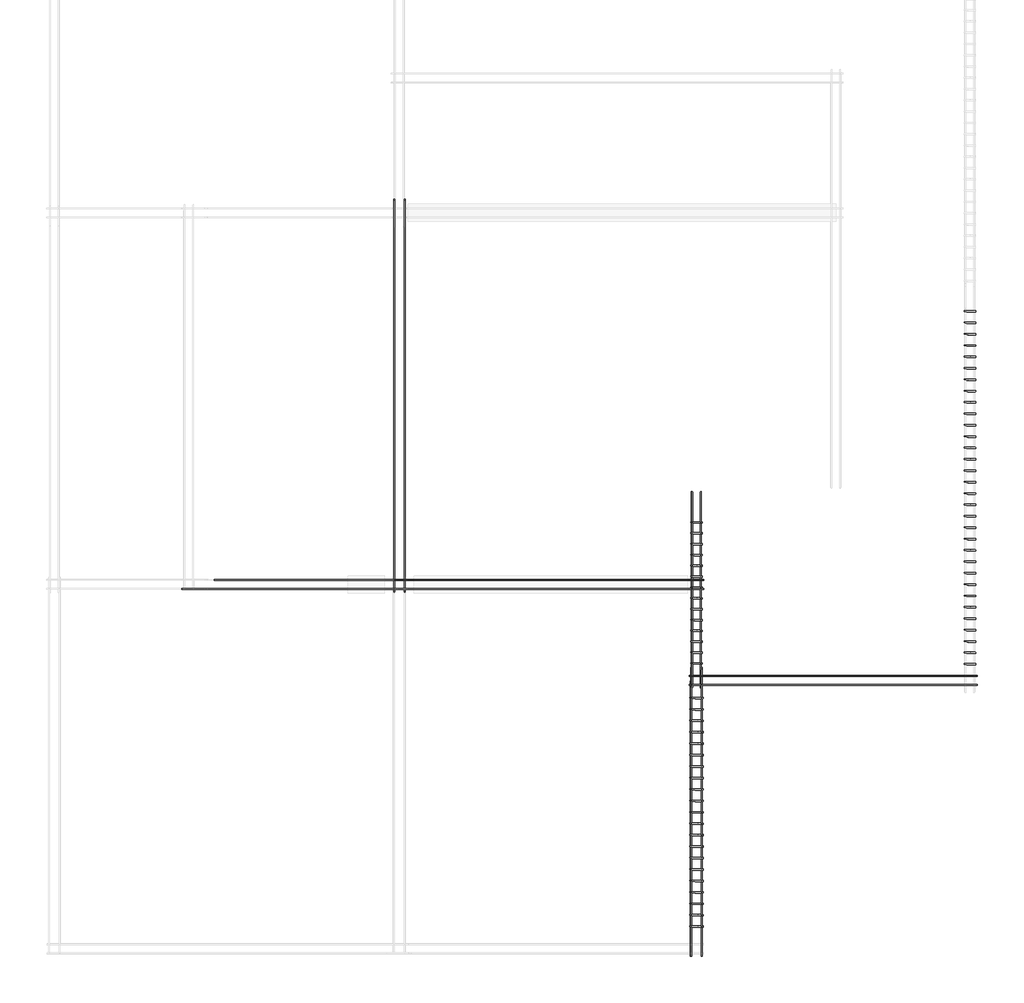
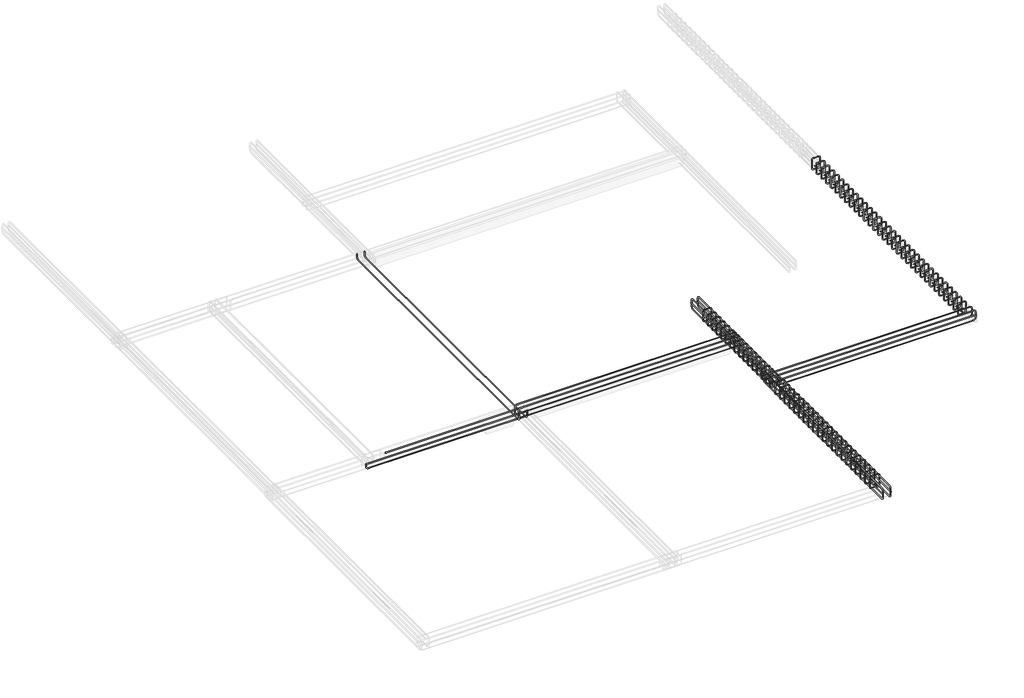
# One storey, part 3 of 5: 32 reinforcing bars.
"""IFC4 building model written with IfcOpenShell, lengths in millimetres."""

from ifc_helpers import new_model, si_unit, point, frame, origin, place, context, project, spatial, polyline, circle_curve, trimmed, segment, composite_curve, source, transform, mapped, element, save
from ifc_brep_helpers import swept_disk

model = new_model("IFC4")

# Units and contexts
model_context = context("Model", 3, world=origin())
ifc_project = project(units=[si_unit("LENGTHUNIT", "METRE", prefix="MILLI")], contexts=[model_context])

# Site, building, storey
site = spatial("IfcSite", under=ifc_project)
building = spatial("IfcBuilding", under=site)
storey = spatial("IfcBuildingStorey", under=building, Elevation=0.0)

# Reinforcing bars
placement = place(None, origin())
element("IfcReinforcingBar", 1, at=placement, inside=storey, context=model_context, shape_type="SolidModel", body=[
    swept_disk(composite_curve([segment(polyline([(-6222.6200976, 4871.519882, 305.3447439), (-6222.6200976, 4871.519882, 254.5447439)]), True, "CONTINUOUS"), segment(trimmed(circle_curve(frame((-6267.0700976, 4871.519882, 254.5447439), z_axis=(0.0, 1.0, 0.0), x_axis=(44.44999999999982, 0.0, 0.0)), 44.45), [point((-6222.6200976, 4871.519882, 254.5447439))], [point((-6267.0700976, 4871.519882, 210.0947439))], True, "CARTESIAN"), True, "CONTINUOUS"), segment(polyline([(-6267.0700976, 4871.519882, 210.0947439), (-10213.1612792, 4871.519882, 210.0947439)]), True, "CONTINUOUS"), segment(trimmed(circle_curve(frame((-10213.1612792, 4871.519882, 254.5447439), z_axis=(0.0, 1.0, 0.0), x_axis=(0.0, 0.0, -44.44999999999999)), 44.45), [point((-10213.1612792, 4871.519882, 210.0947439))], [point((-10257.6112792, 4871.519882, 254.5447439))], True, "CARTESIAN"), True, "CONTINUOUS"), segment(polyline([(-10257.6112792, 4871.519882, 254.5447439), (-10257.6112792, 4871.519882, 305.3447439)]), True, "CONTINUOUS")], self_intersect=False), 6.35),
])
element("IfcReinforcingBar", 2, at=placement, inside=storey, context=model_context, shape_type="SolidModel", body=[
    swept_disk(composite_curve([segment(polyline([(-10091.1292762, 4988.4501382, 304.8), (-12623.4418223, 4988.4501382, 304.8)]), True, "CONTINUOUS")], self_intersect=False), 6.35),
])
element("IfcReinforcingBar", 3, at=placement, inside=storey, context=model_context, shape_type="SolidModel", body=[
    swept_disk(composite_curve([segment(polyline([(-10099.5620565, 4867.8001382, 304.8), (-13051.6902836, 4867.8001382, 304.8)]), True, "CONTINUOUS")], self_intersect=False), 6.35),
])
element("IfcReinforcingBar", 4, at=placement, inside=storey, context=model_context, shape_type="SolidModel", body=[
    swept_disk(composite_curve([segment(polyline([(-6221.7854997, 4984.7303943, 304.2552561), (-6221.7854997, 4984.7303943, 355.0552561)]), True, "CONTINUOUS"), segment(trimmed(circle_curve(frame((-6266.2354997, 4984.7303943, 355.0552561), z_axis=(0.0, -1.0, 0.0), x_axis=(44.44999999999982, 0.0, 0.0)), 44.45), [point((-6221.7854997, 4984.7303943, 355.0552561))], [point((-6266.2354997, 4984.7303943, 399.5052561))], True, "CARTESIAN"), True, "CONTINUOUS"), segment(polyline([(-6266.2354997, 4984.7303943, 399.5052561), (-10213.1612792, 4984.7303943, 399.5052561)]), True, "CONTINUOUS"), segment(trimmed(circle_curve(frame((-10213.1612792, 4984.7303943, 355.0552561), z_axis=(0.0, -1.0, 0.0), x_axis=(0.0, 0.0, 44.44999999999999)), 44.45), [point((-10213.1612792, 4984.7303943, 399.5052561))], [point((-10257.6112792, 4984.7303943, 355.0552561))], True, "CARTESIAN"), True, "CONTINUOUS"), segment(polyline([(-10257.6112792, 4984.7303943, 355.0552561), (-10257.6112792, 4984.7303943, 304.2552561)]), True, "CONTINUOUS")], self_intersect=False), 6.35),
])
element("IfcReinforcingBar", 5, at=placement, inside=storey, context=model_context, shape_type="SolidModel", body=[
    swept_disk(composite_curve([segment(polyline([(-6222.3875013, 4871.519882, 304.2552561), (-6222.3875013, 4871.519882, 355.0552561)]), True, "CONTINUOUS"), segment(trimmed(circle_curve(frame((-6266.8375013, 4871.519882, 355.0552561), z_axis=(0.0, -1.0, 0.0), x_axis=(44.45000000000073, 0.0, 0.0)), 44.45), [point((-6222.3875013, 4871.519882, 355.0552561))], [point((-6266.8375013, 4871.519882, 399.5052561))], True, "CARTESIAN"), True, "CONTINUOUS"), segment(polyline([(-6266.8375013, 4871.519882, 399.5052561), (-10213.3791411, 4871.519882, 399.5052561)]), True, "CONTINUOUS"), segment(trimmed(circle_curve(frame((-10213.3791411, 4871.519882, 355.0552561), z_axis=(0.0, -1.0, 0.0), x_axis=(0.0, 0.0, 44.44999999999999)), 44.45), [point((-10213.3791411, 4871.519882, 399.5052561))], [point((-10257.8291411, 4871.519882, 355.0552561))], True, "CARTESIAN"), True, "CONTINUOUS"), segment(polyline([(-10257.8291411, 4871.519882, 355.0552561), (-10257.8291411, 4871.519882, 304.2552561)]), True, "CONTINUOUS")], self_intersect=False), 6.35),
])
element("IfcReinforcingBar", 6, at=placement, inside=storey, context=model_context, shape_type="SolidModel", body=[
    swept_disk(composite_curve([segment(polyline([(-6222.9639641, 4984.7303943, 305.3447439), (-6222.9639641, 4984.7303943, 254.5447439)]), True, "CONTINUOUS"), segment(trimmed(circle_curve(frame((-6267.4139641, 4984.7303943, 254.5447439), z_axis=(0.0, 1.0, 0.0), x_axis=(44.44999999999982, 0.0, 0.0)), 44.45), [point((-6222.9639641, 4984.7303943, 254.5447439))], [point((-6267.4139641, 4984.7303943, 210.0947439))], True, "CARTESIAN"), True, "CONTINUOUS"), segment(polyline([(-6267.4139641, 4984.7303943, 210.0947439), (-10213.8368777, 4984.7303943, 210.0947439)]), True, "CONTINUOUS"), segment(trimmed(circle_curve(frame((-10213.8368777, 4984.7303943, 254.5447439), z_axis=(0.0, 1.0, 0.0), x_axis=(0.0, 0.0, -44.44999999999999)), 44.45), [point((-10213.8368777, 4984.7303943, 210.0947439))], [point((-10258.2868777, 4984.7303943, 254.5447439))], True, "CARTESIAN"), True, "CONTINUOUS"), segment(polyline([(-10258.2868777, 4984.7303943, 254.5447439), (-10258.2868777, 4984.7303943, 305.3447439)]), True, "CONTINUOUS")], self_intersect=False), 6.35),
])
element("IfcReinforcingBar", 7, at=placement, inside=storey, context=model_context, shape_type="SolidModel", body=[
    swept_disk(composite_curve([segment(polyline([(-10095.8173663, 4871.519882, 305.3447439), (-10095.8173663, 4871.519882, 254.5447439)]), True, "CONTINUOUS"), segment(trimmed(circle_curve(frame((-10140.2673663, 4871.519882, 254.5447439), z_axis=(0.0, 1.0, 0.0), x_axis=(44.45000000000073, 0.0, 0.0)), 44.45), [point((-10095.8173663, 4871.519882, 254.5447439))], [point((-10140.2673663, 4871.519882, 210.0947439))], True, "CARTESIAN"), True, "CONTINUOUS"), segment(polyline([(-10140.2673663, 4871.519882, 210.0947439), (-13000.8038783, 4871.519882, 210.0947439)]), True, "CONTINUOUS"), segment(trimmed(circle_curve(frame((-13000.8038783, 4871.519882, 254.5447439), z_axis=(0.0, 1.0, 0.0), x_axis=(0.0, 0.0, -44.44999999999999)), 44.45), [point((-13000.8038783, 4871.519882, 210.0947439))], [point((-13045.2538783, 4871.519882, 254.5447439))], True, "CARTESIAN"), True, "CONTINUOUS"), segment(polyline([(-13045.2538783, 4871.519882, 254.5447439), (-13045.2538783, 4871.519882, 305.3447439)]), True, "CONTINUOUS")], self_intersect=False), 6.35),
])
element("IfcReinforcingBar", 8, at=placement, inside=storey, context=model_context, shape_type="SolidModel", body=[
    swept_disk(composite_curve([segment(polyline([(-6216.0848989, 4988.4501382, 304.8), (-10264.974677, 4988.4501382, 304.8)]), True, "CONTINUOUS")], self_intersect=False), 6.35),
])
element("IfcReinforcingBar", 9, at=placement, inside=storey, context=model_context, shape_type="SolidModel", body=[
    swept_disk(composite_curve([segment(polyline([(-6215.9707513, 4867.8001382, 304.8), (-10257.7161484, 4867.8001382, 304.8)]), True, "CONTINUOUS")], self_intersect=False), 6.35),
])
reinforcing_bar_shape = source(origin(), model_context, "Body", "SolidModel", [
    swept_disk(composite_curve([segment(polyline([(-6291.2430392, 451.8078802, 280.0771773), (-6234.3788421, 451.8078802, 223.2129802)]), True, "CONTINUOUS"), segment(trimmed(circle_curve(frame((-6251.2168223, 451.8078802, 206.375), z_axis=(0.0, 1.0, 0.0), x_axis=(16.837980199999947, 0.0, 16.837980200000004)), 23.8125), [point((-6234.3788421, 451.8078802, 223.2129802))], [point((-6251.2168223, 451.8078802, 182.5625))], True, "CARTESIAN"), True, "CONTINUOUS"), segment(polyline([(-6251.2168223, 451.8078802, 182.5625), (-6371.8668223, 451.8078802, 182.5625)]), True, "CONTINUOUS"), segment(trimmed(circle_curve(frame((-6371.8668223, 451.8078802, 206.375), z_axis=(0.0, 1.0, 0.0), x_axis=(0.0, 0.0, -23.8125)), 23.8125), [point((-6371.8668223, 451.8078802, 182.5625))], [point((-6395.6793223, 451.8078802, 206.375))], True, "CARTESIAN"), True, "CONTINUOUS"), segment(polyline([(-6395.6793223, 451.8078802, 206.375), (-6395.6793223, 451.8078802, 390.525)]), True, "CONTINUOUS"), segment(trimmed(circle_curve(frame((-6371.9048784, 450.4621569, 390.525), z_axis=(0.056513312022652806, 0.9984018457335856, 0.0), x_axis=(-23.774443900000733, 1.3457232999999746, 0.0)), 23.8125), [point((-6395.6793223, 451.8078802, 390.525))], [point((-6371.9048784, 450.4621569, 414.3375))], True, "CARTESIAN"), True, "CONTINUOUS"), segment(polyline([(-6371.9048784, 450.4621569, 414.3375), (-6251.1787663, 443.6286034, 414.3375)]), True, "CONTINUOUS"), segment(trimmed(circle_curve(frame((-6251.1787663, 443.6286034, 390.525), z_axis=(0.0565133120226528, 0.9984018457335855, 0.0), x_axis=(0.0, 0.0, 23.8125)), 23.8125), [point((-6251.1787663, 443.6286034, 414.3375))], [point((-6227.4043223, 442.2828802, 390.525))], True, "CARTESIAN"), True, "CONTINUOUS"), segment(polyline([(-6227.4043223, 442.2828802, 390.525), (-6227.4043223, 442.2828802, 206.375)]), True, "CONTINUOUS"), segment(trimmed(circle_curve(frame((-6251.2168223, 442.2828802, 206.375), z_axis=(0.0, 1.0, 0.0), x_axis=(23.8125, 0.0, 0.0)), 23.8125), [point((-6227.4043223, 442.2828802, 206.375))], [point((-6268.0548025, 442.2828802, 189.5370198))], True, "CARTESIAN"), True, "CONTINUOUS"), segment(polyline([(-6268.0548025, 442.2828802, 189.5370198), (-6324.9189996, 442.2828802, 246.4012168)]), True, "CONTINUOUS")], self_intersect=False), 4.7625),
])
element("IfcReinforcingBar", 10, at=placement, inside=storey, context=model_context, shape_type="MappedRepresentation", body=[
    mapped(reinforcing_bar_shape, transform((0.0, 0.0, 0.0), x_axis=(1.0, 0.0, 0.0), y_axis=(0.0, 1.0, 0.0), z_axis=(0.0, 0.0, 1.0))),
    mapped(reinforcing_bar_shape, transform((0.0, 149.7514784, 0.0), x_axis=(1.0, 0.0, 0.0), y_axis=(0.0, 1.0, 0.0), z_axis=(0.0, 0.0, 1.0))),
    mapped(reinforcing_bar_shape, transform((0.0, 299.5029567, 0.0), x_axis=(1.0, 0.0, 0.0), y_axis=(0.0, 1.0, 0.0), z_axis=(0.0, 0.0, 1.0))),
    mapped(reinforcing_bar_shape, transform((0.0, 449.2544351, 0.0), x_axis=(1.0, 0.0, 0.0), y_axis=(0.0, 1.0, 0.0), z_axis=(0.0, 0.0, 1.0))),
    mapped(reinforcing_bar_shape, transform((0.0, 599.0059134, 0.0), x_axis=(1.0, 0.0, 0.0), y_axis=(0.0, 1.0, 0.0), z_axis=(0.0, 0.0, 1.0))),
    mapped(reinforcing_bar_shape, transform((0.0, 748.7573918, 0.0), x_axis=(1.0, 0.0, 0.0), y_axis=(0.0, 1.0, 0.0), z_axis=(0.0, 0.0, 1.0))),
    mapped(reinforcing_bar_shape, transform((0.0, 898.5088701, 0.0), x_axis=(1.0, 0.0, 0.0), y_axis=(0.0, 1.0, 0.0), z_axis=(0.0, 0.0, 1.0))),
    mapped(reinforcing_bar_shape, transform((0.0, 1048.2603485, 0.0), x_axis=(1.0, 0.0, 0.0), y_axis=(0.0, 1.0, 0.0), z_axis=(0.0, 0.0, 1.0))),
    mapped(reinforcing_bar_shape, transform((0.0, 1198.0118268, 0.0), x_axis=(1.0, 0.0, 0.0), y_axis=(0.0, 1.0, 0.0), z_axis=(0.0, 0.0, 1.0))),
    mapped(reinforcing_bar_shape, transform((0.0, 1347.7633052, 0.0), x_axis=(1.0, 0.0, 0.0), y_axis=(0.0, 1.0, 0.0), z_axis=(0.0, 0.0, 1.0))),
    mapped(reinforcing_bar_shape, transform((0.0, 1497.5147835, 0.0), x_axis=(1.0, 0.0, 0.0), y_axis=(0.0, 1.0, 0.0), z_axis=(0.0, 0.0, 1.0))),
    mapped(reinforcing_bar_shape, transform((0.0, 1647.2662619, 0.0), x_axis=(1.0, 0.0, 0.0), y_axis=(0.0, 1.0, 0.0), z_axis=(0.0, 0.0, 1.0))),
    mapped(reinforcing_bar_shape, transform((0.0, 1797.0177402, 0.0), x_axis=(1.0, 0.0, 0.0), y_axis=(0.0, 1.0, 0.0), z_axis=(0.0, 0.0, 1.0))),
    mapped(reinforcing_bar_shape, transform((0.0, 1946.7692186, 0.0), x_axis=(1.0, 0.0, 0.0), y_axis=(0.0, 1.0, 0.0), z_axis=(0.0, 0.0, 1.0))),
    mapped(reinforcing_bar_shape, transform((0.0, 2096.5206969, 0.0), x_axis=(1.0, 0.0, 0.0), y_axis=(0.0, 1.0, 0.0), z_axis=(0.0, 0.0, 1.0))),
    mapped(reinforcing_bar_shape, transform((0.0, 2246.2721753, 0.0), x_axis=(1.0, 0.0, 0.0), y_axis=(0.0, 1.0, 0.0), z_axis=(0.0, 0.0, 1.0))),
    mapped(reinforcing_bar_shape, transform((0.0, 2396.0236537, 0.0), x_axis=(1.0, 0.0, 0.0), y_axis=(0.0, 1.0, 0.0), z_axis=(0.0, 0.0, 1.0))),
    mapped(reinforcing_bar_shape, transform((0.0, 2545.775132, 0.0), x_axis=(1.0, 0.0, 0.0), y_axis=(0.0, 1.0, 0.0), z_axis=(0.0, 0.0, 1.0))),
    mapped(reinforcing_bar_shape, transform((0.0, 2695.5266104, 0.0), x_axis=(1.0, 0.0, 0.0), y_axis=(0.0, 1.0, 0.0), z_axis=(0.0, 0.0, 1.0))),
    mapped(reinforcing_bar_shape, transform((0.0, 2845.2780887, 0.0), x_axis=(1.0, 0.0, 0.0), y_axis=(0.0, 1.0, 0.0), z_axis=(0.0, 0.0, 1.0))),
    mapped(reinforcing_bar_shape, transform((0.0, 2995.0295671, 0.0), x_axis=(1.0, 0.0, 0.0), y_axis=(0.0, 1.0, 0.0), z_axis=(0.0, 0.0, 1.0))),
])
element("IfcReinforcingBar", 11, at=placement, inside=storey, context=model_context, shape_type="SolidModel", body=[
    swept_disk(composite_curve([segment(polyline([(-6242.2365662, 63.6013487, 304.2552561), (-6242.2365662, 63.6013487, 355.0552561)]), True, "CONTINUOUS"), segment(trimmed(circle_curve(frame((-6242.2365662, 108.0513487, 355.0552561), z_axis=(-1.0, 0.0, 0.0), x_axis=(0.0, -44.45, 0.0)), 44.45), [point((-6242.2365662, 63.6013487, 355.0552561))], [point((-6242.2365662, 108.0513487, 399.5052561))], True, "CARTESIAN"), True, "CONTINUOUS"), segment(polyline([(-6242.2365662, 108.0513487, 399.5052561), (-6242.2365662, 3794.9070918, 399.5052561)]), True, "CONTINUOUS"), segment(trimmed(circle_curve(frame((-6242.2365662, 3794.9070918, 355.0552561), z_axis=(-1.0, 0.0, 0.0), x_axis=(0.0, 0.0, 44.44999999999999)), 44.45), [point((-6242.2365662, 3794.9070918, 399.5052561))], [point((-6242.2365662, 3839.3570918, 355.0552561))], True, "CARTESIAN"), True, "CONTINUOUS"), segment(polyline([(-6242.2365662, 3839.3570918, 355.0552561), (-6242.2365662, 3839.3570918, 304.2552561)]), True, "CONTINUOUS")], self_intersect=False), 6.35),
])
element("IfcReinforcingBar", 12, at=placement, inside=storey, context=model_context, shape_type="SolidModel", body=[
    swept_disk(composite_curve([segment(polyline([(-6380.8470784, 64.2033502, 304.2552561), (-6380.8470784, 64.2033502, 355.0552561)]), True, "CONTINUOUS"), segment(trimmed(circle_curve(frame((-6380.8470784, 108.6533502, 355.0552561), z_axis=(-1.0, 0.0, 0.0), x_axis=(0.0, -44.45, 0.0)), 44.45), [point((-6380.8470784, 64.2033502, 355.0552561))], [point((-6380.8470784, 108.6533502, 399.5052561))], True, "CARTESIAN"), True, "CONTINUOUS"), segment(polyline([(-6380.8470784, 108.6533502, 399.5052561), (-6380.8470784, 3794.8108119, 399.5052561)]), True, "CONTINUOUS"), segment(trimmed(circle_curve(frame((-6380.8470784, 3794.8108119, 355.0552561), z_axis=(-1.0, 0.0, 0.0), x_axis=(0.0, 0.0, 44.44999999999999)), 44.45), [point((-6380.8470784, 3794.8108119, 399.5052561))], [point((-6380.8470784, 3839.2608119, 355.0552561))], True, "CARTESIAN"), True, "CONTINUOUS"), segment(polyline([(-6380.8470784, 3839.2608119, 355.0552561), (-6380.8470784, 3839.2608119, 304.2552561)]), True, "CONTINUOUS")], self_intersect=False), 6.35),
])
element("IfcReinforcingBar", 13, at=placement, inside=storey, context=model_context, shape_type="SolidModel", body=[
    swept_disk(composite_curve([segment(polyline([(-6242.2365662, 64.7798131, 292.6447439), (-6242.2365662, 64.7798131, 241.8447439)]), True, "CONTINUOUS"), segment(trimmed(circle_curve(frame((-6242.2365662, 109.2298131, 241.8447439), z_axis=(1.0, 0.0, 0.0), x_axis=(0.0, -44.45, 0.0)), 44.45), [point((-6242.2365662, 64.7798131, 241.8447439))], [point((-6242.2365662, 109.2298131, 197.3947439))], True, "CARTESIAN"), True, "CONTINUOUS"), segment(polyline([(-6242.2365662, 109.2298131, 197.3947439), (-6242.2365662, 3794.6550905, 197.3947439)]), True, "CONTINUOUS"), segment(trimmed(circle_curve(frame((-6242.2365662, 3794.6550905, 241.8447439), z_axis=(1.0, 0.0, 0.0), x_axis=(0.0, 0.0, -44.44999999999999)), 44.45), [point((-6242.2365662, 3794.6550905, 197.3947439))], [point((-6242.2365662, 3839.1050905, 241.8447439))], True, "CARTESIAN"), True, "CONTINUOUS"), segment(polyline([(-6242.2365662, 3839.1050905, 241.8447439), (-6242.2365662, 3839.1050905, 292.6447439)]), True, "CONTINUOUS")], self_intersect=False), 6.35),
])
element("IfcReinforcingBar", 14, at=placement, inside=storey, context=model_context, shape_type="SolidModel", body=[
    swept_disk(composite_curve([segment(polyline([(-6380.8470784, 65.0583978, 292.6447439), (-6380.8470784, 65.0583978, 241.8447439)]), True, "CONTINUOUS"), segment(trimmed(circle_curve(frame((-6380.8470784, 109.5083978, 241.8447439), z_axis=(1.0, 0.0, 0.0), x_axis=(0.0, -44.45, 0.0)), 44.45), [point((-6380.8470784, 65.0583978, 241.8447439))], [point((-6380.8470784, 109.5083978, 197.3947439))], True, "CARTESIAN"), True, "CONTINUOUS"), segment(polyline([(-6380.8470784, 109.5083978, 197.3947439), (-6380.8470784, 3794.2868584, 197.3947439)]), True, "CONTINUOUS"), segment(trimmed(circle_curve(frame((-6380.8470784, 3794.2868584, 241.8447439), z_axis=(1.0, 0.0, 0.0), x_axis=(0.0, 0.0, -44.44999999999999)), 44.45), [point((-6380.8470784, 3794.2868584, 197.3947439))], [point((-6380.8470784, 3838.7368584, 241.8447439))], True, "CARTESIAN"), True, "CONTINUOUS"), segment(polyline([(-6380.8470784, 3838.7368584, 241.8447439), (-6380.8470784, 3838.7368584, 292.6447439)]), True, "CONTINUOUS")], self_intersect=False), 6.35),
])
element("IfcReinforcingBar", 15, at=placement, inside=storey, context=model_context, shape_type="SolidModel", body=[
    swept_disk(composite_curve([segment(polyline([(-6238.5168223, 57.9007478, 304.8), (-6238.5168223, 3806.0293558, 304.8)]), True, "CONTINUOUS")], self_intersect=False), 6.35),
])
element("IfcReinforcingBar", 16, at=placement, inside=storey, context=model_context, shape_type="SolidModel", body=[
    swept_disk(composite_curve([segment(polyline([(-6384.5668223, 57.7866002, 304.8), (-6384.5668223, 3664.7531365, 304.8)]), True, "CONTINUOUS")], self_intersect=False), 6.35),
])
reinforcing_bar_2_shape = source(origin(), model_context, "Body", "SolidModel", [
    swept_disk(composite_curve([segment(polyline([(-6303.9430392, 3899.4936519, 292.7771773), (-6247.0788421, 3899.4936519, 235.9129802)]), True, "CONTINUOUS"), segment(trimmed(circle_curve(frame((-6263.9168223, 3899.4936519, 219.075), z_axis=(0.0, 1.0, 0.0), x_axis=(16.837980199999947, 0.0, 16.837980200000004)), 23.8125), [point((-6247.0788421, 3899.4936519, 235.9129802))], [point((-6263.9168223, 3899.4936519, 195.2625))], True, "CARTESIAN"), True, "CONTINUOUS"), segment(polyline([(-6263.9168223, 3899.4936519, 195.2625), (-6359.1668223, 3899.4936519, 195.2625)]), True, "CONTINUOUS"), segment(trimmed(circle_curve(frame((-6359.1668223, 3899.4936519, 219.075), z_axis=(0.0, 1.0, 0.0), x_axis=(0.0, 0.0, -23.8125)), 23.8125), [point((-6359.1668223, 3899.4936519, 195.2625))], [point((-6382.9793223, 3899.4936519, 219.075))], True, "CARTESIAN"), True, "CONTINUOUS"), segment(polyline([(-6382.9793223, 3899.4936519, 219.075), (-6382.9793223, 3899.4936519, 390.525)]), True, "CONTINUOUS"), segment(trimmed(circle_curve(frame((-6359.2195633, 3897.9096679, 390.525), z_axis=(0.06651901052377011, 0.9977851578566093, 0.0), x_axis=(-23.759758999999576, 1.583983999999873, 0.0)), 23.8125), [point((-6382.9793223, 3899.4936519, 390.525))], [point((-6359.2195633, 3897.9096679, 414.3375))], True, "CARTESIAN"), True, "CONTINUOUS"), segment(polyline([(-6359.2195633, 3897.9096679, 414.3375), (-6263.8640814, 3891.5526358, 414.3375)]), True, "CONTINUOUS"), segment(trimmed(circle_curve(frame((-6263.8640814, 3891.5526358, 390.525), z_axis=(0.06651901052377011, 0.9977851578566093, 0.0), x_axis=(0.0, 0.0, 23.8125)), 23.8125), [point((-6263.8640814, 3891.5526358, 414.3375))], [point((-6240.1043223, 3889.9686519, 390.525))], True, "CARTESIAN"), True, "CONTINUOUS"), segment(polyline([(-6240.1043223, 3889.9686519, 390.525), (-6240.1043223, 3889.9686519, 219.075)]), True, "CONTINUOUS"), segment(trimmed(circle_curve(frame((-6263.9168223, 3889.9686519, 219.075), z_axis=(0.0, 1.0, 0.0), x_axis=(23.8125, 0.0, 0.0)), 23.8125), [point((-6240.1043223, 3889.9686519, 219.075))], [point((-6280.7548025, 3889.9686519, 202.2370198))], True, "CARTESIAN"), True, "CONTINUOUS"), segment(polyline([(-6280.7548025, 3889.9686519, 202.2370198), (-6337.6189996, 3889.9686519, 259.1012168)]), True, "CONTINUOUS")], self_intersect=False), 4.7625),
])
element("IfcReinforcingBar", 17, at=placement, inside=storey, context=model_context, shape_type="MappedRepresentation", body=[
    mapped(reinforcing_bar_2_shape, transform((0.0, 0.0, 0.0), x_axis=(1.0, 0.0, 0.0), y_axis=(0.0, 1.0, 0.0), z_axis=(0.0, 0.0, 1.0))),
    mapped(reinforcing_bar_2_shape, transform((0.0, 142.0033689, 0.0), x_axis=(1.0, 0.0, 0.0), y_axis=(0.0, 1.0, 0.0), z_axis=(0.0, 0.0, 1.0))),
    mapped(reinforcing_bar_2_shape, transform((0.0, 284.0067377, 0.0), x_axis=(1.0, 0.0, 0.0), y_axis=(0.0, 1.0, 0.0), z_axis=(0.0, 0.0, 1.0))),
    mapped(reinforcing_bar_2_shape, transform((0.0, 426.0101066, 0.0), x_axis=(1.0, 0.0, 0.0), y_axis=(0.0, 1.0, 0.0), z_axis=(0.0, 0.0, 1.0))),
    mapped(reinforcing_bar_2_shape, transform((0.0, 568.0134755, 0.0), x_axis=(1.0, 0.0, 0.0), y_axis=(0.0, 1.0, 0.0), z_axis=(0.0, 0.0, 1.0))),
    mapped(reinforcing_bar_2_shape, transform((0.0, 710.0168444, 0.0), x_axis=(1.0, 0.0, 0.0), y_axis=(0.0, 1.0, 0.0), z_axis=(0.0, 0.0, 1.0))),
    mapped(reinforcing_bar_2_shape, transform((0.0, 852.0202132, 0.0), x_axis=(1.0, 0.0, 0.0), y_axis=(0.0, 1.0, 0.0), z_axis=(0.0, 0.0, 1.0))),
    mapped(reinforcing_bar_2_shape, transform((0.0, 994.0235821, 0.0), x_axis=(1.0, 0.0, 0.0), y_axis=(0.0, 1.0, 0.0), z_axis=(0.0, 0.0, 1.0))),
    mapped(reinforcing_bar_2_shape, transform((0.0, 1136.026951, 0.0), x_axis=(1.0, 0.0, 0.0), y_axis=(0.0, 1.0, 0.0), z_axis=(0.0, 0.0, 1.0))),
    mapped(reinforcing_bar_2_shape, transform((0.0, 1278.0303199, 0.0), x_axis=(1.0, 0.0, 0.0), y_axis=(0.0, 1.0, 0.0), z_axis=(0.0, 0.0, 1.0))),
    mapped(reinforcing_bar_2_shape, transform((0.0, 1420.0336887, 0.0), x_axis=(1.0, 0.0, 0.0), y_axis=(0.0, 1.0, 0.0), z_axis=(0.0, 0.0, 1.0))),
    mapped(reinforcing_bar_2_shape, transform((0.0, 1562.0370576, 0.0), x_axis=(1.0, 0.0, 0.0), y_axis=(0.0, 1.0, 0.0), z_axis=(0.0, 0.0, 1.0))),
    mapped(reinforcing_bar_2_shape, transform((0.0, 1704.0404265, 0.0), x_axis=(1.0, 0.0, 0.0), y_axis=(0.0, 1.0, 0.0), z_axis=(0.0, 0.0, 1.0))),
    mapped(reinforcing_bar_2_shape, transform((0.0, 1846.0437954, 0.0), x_axis=(1.0, 0.0, 0.0), y_axis=(0.0, 1.0, 0.0), z_axis=(0.0, 0.0, 1.0))),
])
element("IfcReinforcingBar", 18, at=placement, inside=storey, context=model_context, shape_type="SolidModel", body=[
    swept_disk(composite_curve([segment(polyline([(-6254.9365662, 3581.5015576, 304.2552561), (-6254.9365662, 3581.5015576, 355.0552561)]), True, "CONTINUOUS"), segment(trimmed(circle_curve(frame((-6254.9365662, 3625.9515576, 355.0552561), z_axis=(-1.0, 0.0, 0.0), x_axis=(0.0, -44.44999999999982, 0.0)), 44.45), [point((-6254.9365662, 3581.5015576, 355.0552561))], [point((-6254.9365662, 3625.9515576, 399.5052561))], True, "CARTESIAN"), True, "CONTINUOUS"), segment(polyline([(-6254.9365662, 3625.9515576, 399.5052561), (-6254.9365662, 6093.6070918, 399.5052561)]), True, "CONTINUOUS"), segment(trimmed(circle_curve(frame((-6254.9365662, 6093.6070918, 355.0552561), z_axis=(-1.0, 0.0, 0.0), x_axis=(0.0, 0.0, 44.44999999999999)), 44.45), [point((-6254.9365662, 6093.6070918, 399.5052561))], [point((-6254.9365662, 6138.0570918, 355.0552561))], True, "CARTESIAN"), True, "CONTINUOUS"), segment(polyline([(-6254.9365662, 6138.0570918, 355.0552561), (-6254.9365662, 6138.0570918, 304.2552561)]), True, "CONTINUOUS")], self_intersect=False), 6.35),
])
element("IfcReinforcingBar", 19, at=placement, inside=storey, context=model_context, shape_type="SolidModel", body=[
    swept_disk(composite_curve([segment(polyline([(-6368.1470784, 3582.1035591, 304.2552561), (-6368.1470784, 3582.1035591, 355.0552561)]), True, "CONTINUOUS"), segment(trimmed(circle_curve(frame((-6368.1470784, 3626.5535591, 355.0552561), z_axis=(-1.0, 0.0, 0.0), x_axis=(0.0, -44.44999999999982, 0.0)), 44.45), [point((-6368.1470784, 3582.1035591, 355.0552561))], [point((-6368.1470784, 3626.5535591, 399.5052561))], True, "CARTESIAN"), True, "CONTINUOUS"), segment(polyline([(-6368.1470784, 3626.5535591, 399.5052561), (-6368.1470784, 6093.5108119, 399.5052561)]), True, "CONTINUOUS"), segment(trimmed(circle_curve(frame((-6368.1470784, 6093.5108119, 355.0552561), z_axis=(-1.0, 0.0, 0.0), x_axis=(0.0, 0.0, 44.44999999999999)), 44.45), [point((-6368.1470784, 6093.5108119, 399.5052561))], [point((-6368.1470784, 6137.9608119, 355.0552561))], True, "CARTESIAN"), True, "CONTINUOUS"), segment(polyline([(-6368.1470784, 6137.9608119, 355.0552561), (-6368.1470784, 6137.9608119, 304.2552561)]), True, "CONTINUOUS")], self_intersect=False), 6.35),
])
element("IfcReinforcingBar", 20, at=placement, inside=storey, context=model_context, shape_type="SolidModel", body=[
    swept_disk(composite_curve([segment(polyline([(-6254.9365662, 3582.680022, 305.3447439), (-6254.9365662, 3582.680022, 254.5447439)]), True, "CONTINUOUS"), segment(trimmed(circle_curve(frame((-6254.9365662, 3627.130022, 254.5447439), z_axis=(1.0, 0.0, 0.0), x_axis=(0.0, -44.44999999999982, 0.0)), 44.45), [point((-6254.9365662, 3582.680022, 254.5447439))], [point((-6254.9365662, 3627.130022, 210.0947439))], True, "CARTESIAN"), True, "CONTINUOUS"), segment(polyline([(-6254.9365662, 3627.130022, 210.0947439), (-6254.9365662, 6093.3550905, 210.0947439)]), True, "CONTINUOUS"), segment(trimmed(circle_curve(frame((-6254.9365662, 6093.3550905, 254.5447439), z_axis=(1.0, 0.0, 0.0), x_axis=(0.0, 0.0, -44.44999999999999)), 44.45), [point((-6254.9365662, 6093.3550905, 210.0947439))], [point((-6254.9365662, 6137.8050905, 254.5447439))], True, "CARTESIAN"), True, "CONTINUOUS"), segment(polyline([(-6254.9365662, 6137.8050905, 254.5447439), (-6254.9365662, 6137.8050905, 305.3447439)]), True, "CONTINUOUS")], self_intersect=False), 6.35),
])
element("IfcReinforcingBar", 21, at=placement, inside=storey, context=model_context, shape_type="SolidModel", body=[
    swept_disk(composite_curve([segment(polyline([(-6368.1470784, 3582.9586067, 305.3447439), (-6368.1470784, 3582.9586067, 254.5447439)]), True, "CONTINUOUS"), segment(trimmed(circle_curve(frame((-6368.1470784, 3627.4086067, 254.5447439), z_axis=(1.0, 0.0, 0.0), x_axis=(0.0, -44.44999999999982, 0.0)), 44.45), [point((-6368.1470784, 3582.9586067, 254.5447439))], [point((-6368.1470784, 3627.4086067, 210.0947439))], True, "CARTESIAN"), True, "CONTINUOUS"), segment(polyline([(-6368.1470784, 3627.4086067, 210.0947439), (-6368.1470784, 6092.9868584, 210.0947439)]), True, "CONTINUOUS"), segment(trimmed(circle_curve(frame((-6368.1470784, 6092.9868584, 254.5447439), z_axis=(1.0, 0.0, 0.0), x_axis=(0.0, 0.0, -44.44999999999999)), 44.45), [point((-6368.1470784, 6092.9868584, 210.0947439))], [point((-6368.1470784, 6137.4368584, 254.5447439))], True, "CARTESIAN"), True, "CONTINUOUS"), segment(polyline([(-6368.1470784, 6137.4368584, 254.5447439), (-6368.1470784, 6137.4368584, 305.3447439)]), True, "CONTINUOUS")], self_intersect=False), 6.35),
])
element("IfcReinforcingBar", 22, at=placement, inside=storey, context=model_context, shape_type="SolidModel", body=[
    swept_disk(composite_curve([segment(polyline([(-6251.2168223, 3575.8009567, 304.8), (-6251.2168223, 6144.2893856, 304.8)]), True, "CONTINUOUS")], self_intersect=False), 6.35),
])
element("IfcReinforcingBar", 23, at=placement, inside=storey, context=model_context, shape_type="SolidModel", body=[
    swept_disk(composite_curve([segment(polyline([(-6371.8668223, 3598.7372441, 304.8), (-6371.8668223, 6144.2063415, 304.8)]), True, "CONTINUOUS")], self_intersect=False), 6.35),
])
element("IfcReinforcingBar", 24, at=placement, inside=storey, context=model_context, shape_type="SolidModel", body=[
    swept_disk(composite_curve([segment(polyline([(-6401.2981449, 3614.6526241, 304.2552561), (-6401.2981449, 3614.6526241, 355.0552561)]), True, "CONTINUOUS"), segment(trimmed(circle_curve(frame((-6356.8481449, 3614.6526241, 355.0552561), z_axis=(0.0, 1.0, 0.0), x_axis=(-44.44999999999982, 0.0, 0.0)), 44.45), [point((-6401.2981449, 3614.6526241, 355.0552561))], [point((-6356.8481449, 3614.6526241, 399.5052561))], True, "CARTESIAN"), True, "CONTINUOUS"), segment(polyline([(-6356.8481449, 3614.6526241, 399.5052561), (-2682.6926107, 3614.6526241, 399.5052561)]), True, "CONTINUOUS"), segment(trimmed(circle_curve(frame((-2682.6926107, 3614.6526241, 355.0552561), z_axis=(0.0, 1.0, 0.0), x_axis=(0.0, 0.0, 44.44999999999999)), 44.45), [point((-2682.6926107, 3614.6526241, 399.5052561))], [point((-2638.2426107, 3614.6526241, 355.0552561))], True, "CARTESIAN"), True, "CONTINUOUS"), segment(polyline([(-2638.2426107, 3614.6526241, 355.0552561), (-2638.2426107, 3614.6526241, 304.2552561)]), True, "CONTINUOUS")], self_intersect=False), 6.35),
])
element("IfcReinforcingBar", 25, at=placement, inside=storey, context=model_context, shape_type="SolidModel", body=[
    swept_disk(composite_curve([segment(polyline([(-6400.6961434, 3727.8631363, 304.2552561), (-6400.6961434, 3727.8631363, 355.0552561)]), True, "CONTINUOUS"), segment(trimmed(circle_curve(frame((-6356.2461434, 3727.8631363, 355.0552561), z_axis=(0.0, 1.0, 0.0), x_axis=(-44.45000000000073, 0.0, 0.0)), 44.45), [point((-6400.6961434, 3727.8631363, 355.0552561))], [point((-6356.2461434, 3727.8631363, 399.5052561))], True, "CARTESIAN"), True, "CONTINUOUS"), segment(polyline([(-6356.2461434, 3727.8631363, 399.5052561), (-2682.7888906, 3727.8631363, 399.5052561)]), True, "CONTINUOUS"), segment(trimmed(circle_curve(frame((-2682.7888906, 3727.8631363, 355.0552561), z_axis=(0.0, 1.0, 0.0), x_axis=(0.0, 0.0, 44.44999999999999)), 44.45), [point((-2682.7888906, 3727.8631363, 399.5052561))], [point((-2638.3388906, 3727.8631363, 355.0552561))], True, "CARTESIAN"), True, "CONTINUOUS"), segment(polyline([(-2638.3388906, 3727.8631363, 355.0552561), (-2638.3388906, 3727.8631363, 304.2552561)]), True, "CONTINUOUS")], self_intersect=False), 6.35),
])
element("IfcReinforcingBar", 26, at=placement, inside=storey, context=model_context, shape_type="SolidModel", body=[
    swept_disk(composite_curve([segment(polyline([(-6400.1196805, 3614.6526241, 305.3447439), (-6400.1196805, 3614.6526241, 254.5447439)]), True, "CONTINUOUS"), segment(trimmed(circle_curve(frame((-6355.6696805, 3614.6526241, 254.5447439), z_axis=(0.0, -1.0, 0.0), x_axis=(-44.44999999999982, 0.0, 0.0)), 44.45), [point((-6400.1196805, 3614.6526241, 254.5447439))], [point((-6355.6696805, 3614.6526241, 210.0947439))], True, "CARTESIAN"), True, "CONTINUOUS"), segment(polyline([(-6355.6696805, 3614.6526241, 210.0947439), (-2682.944612, 3614.6526241, 210.0947439)]), True, "CONTINUOUS"), segment(trimmed(circle_curve(frame((-2682.944612, 3614.6526241, 254.5447439), z_axis=(0.0, -1.0, 0.0), x_axis=(0.0, 0.0, -44.44999999999999)), 44.45), [point((-2682.944612, 3614.6526241, 210.0947439))], [point((-2638.494612, 3614.6526241, 254.5447439))], True, "CARTESIAN"), True, "CONTINUOUS"), segment(polyline([(-2638.494612, 3614.6526241, 254.5447439), (-2638.494612, 3614.6526241, 305.3447439)]), True, "CONTINUOUS")], self_intersect=False), 6.35),
])
element("IfcReinforcingBar", 27, at=placement, inside=storey, context=model_context, shape_type="SolidModel", body=[
    swept_disk(composite_curve([segment(polyline([(-6399.8410958, 3727.8631363, 305.3447439), (-6399.8410958, 3727.8631363, 254.5447439)]), True, "CONTINUOUS"), segment(trimmed(circle_curve(frame((-6355.3910958, 3727.8631363, 254.5447439), z_axis=(0.0, -1.0, 0.0), x_axis=(-44.45000000000073, 0.0, 0.0)), 44.45), [point((-6399.8410958, 3727.8631363, 254.5447439))], [point((-6355.3910958, 3727.8631363, 210.0947439))], True, "CARTESIAN"), True, "CONTINUOUS"), segment(polyline([(-6355.3910958, 3727.8631363, 210.0947439), (-2683.3128441, 3727.8631363, 210.0947439)]), True, "CONTINUOUS"), segment(trimmed(circle_curve(frame((-2683.3128441, 3727.8631363, 254.5447439), z_axis=(0.0, -1.0, 0.0), x_axis=(0.0, 0.0, -44.44999999999999)), 44.45), [point((-2683.3128441, 3727.8631363, 210.0947439))], [point((-2638.8628441, 3727.8631363, 254.5447439))], True, "CARTESIAN"), True, "CONTINUOUS"), segment(polyline([(-2638.8628441, 3727.8631363, 254.5447439), (-2638.8628441, 3727.8631363, 305.3447439)]), True, "CONTINUOUS")], self_intersect=False), 6.35),
])
element("IfcReinforcingBar", 28, at=placement, inside=storey, context=model_context, shape_type="SolidModel", body=[
    swept_disk(composite_curve([segment(polyline([(-6406.9987458, 3610.9328802, 304.8), (-2632.5725908, 3610.9328802, 304.8)]), True, "CONTINUOUS")], self_intersect=False), 6.35),
])
element("IfcReinforcingBar", 29, at=placement, inside=storey, context=model_context, shape_type="SolidModel", body=[
    swept_disk(composite_curve([segment(polyline([(-6407.1128934, 3731.5828802, 304.8), (-2632.8065556, 3731.5828802, 304.8)]), True, "CONTINUOUS")], self_intersect=False), 6.35),
])
reinforcing_bar_3_shape = source(origin(), model_context, "Body", "SolidModel", [
    swept_disk(composite_curve([segment(polyline([(-2722.5430392, 3888.6605507, 292.7771773), (-2665.6788421, 3888.6605507, 235.9129802)]), True, "CONTINUOUS"), segment(trimmed(circle_curve(frame((-2682.5168223, 3888.6605507, 219.075), z_axis=(0.0, 1.0, 0.0), x_axis=(16.837980199999947, 0.0, 16.837980200000004)), 23.8125), [point((-2665.6788421, 3888.6605507, 235.9129802))], [point((-2682.5168223, 3888.6605507, 195.2625))], True, "CARTESIAN"), True, "CONTINUOUS"), segment(polyline([(-2682.5168223, 3888.6605507, 195.2625), (-2777.7668223, 3888.6605507, 195.2625)]), True, "CONTINUOUS"), segment(trimmed(circle_curve(frame((-2777.7668223, 3888.6605507, 219.075), z_axis=(0.0, 1.0, 0.0), x_axis=(0.0, 0.0, -23.8125)), 23.8125), [point((-2777.7668223, 3888.6605507, 195.2625))], [point((-2801.5793223, 3888.6605507, 219.075))], True, "CARTESIAN"), True, "CONTINUOUS"), segment(polyline([(-2801.5793223, 3888.6605507, 219.075), (-2801.5793223, 3888.6605507, 390.525)]), True, "CONTINUOUS"), segment(trimmed(circle_curve(frame((-2777.8195633, 3887.0765667, 390.525), z_axis=(0.06651901052377031, 0.9977851578566092, 0.0), x_axis=(-23.75975900000003, 1.583983999999873, 0.0)), 23.8125), [point((-2801.5793223, 3888.6605507, 390.525))], [point((-2777.8195633, 3887.0765667, 414.3375))], True, "CARTESIAN"), True, "CONTINUOUS"), segment(polyline([(-2777.8195633, 3887.0765667, 414.3375), (-2682.4640814, 3880.7195346, 414.3375)]), True, "CONTINUOUS"), segment(trimmed(circle_curve(frame((-2682.4640814, 3880.7195346, 390.525), z_axis=(0.06651901052377031, 0.9977851578566092, 0.0), x_axis=(0.0, 0.0, 23.8125)), 23.8125), [point((-2682.4640814, 3880.7195346, 414.3375))], [point((-2658.7043223, 3879.1355507, 390.525))], True, "CARTESIAN"), True, "CONTINUOUS"), segment(polyline([(-2658.7043223, 3879.1355507, 390.525), (-2658.7043223, 3879.1355507, 219.075)]), True, "CONTINUOUS"), segment(trimmed(circle_curve(frame((-2682.5168223, 3879.1355507, 219.075), z_axis=(0.0, 1.0, 0.0), x_axis=(23.8125, 0.0, 0.0)), 23.8125), [point((-2658.7043223, 3879.1355507, 219.075))], [point((-2699.3548025, 3879.1355507, 202.2370198))], True, "CARTESIAN"), True, "CONTINUOUS"), segment(polyline([(-2699.3548025, 3879.1355507, 202.2370198), (-2756.2189996, 3879.1355507, 259.1012168)]), True, "CONTINUOUS")], self_intersect=False), 4.7625),
])
element("IfcReinforcingBar", 30, at=placement, inside=storey, context=model_context, shape_type="MappedRepresentation", body=[
    mapped(reinforcing_bar_3_shape, transform((0.0, 0.0, 0.0), x_axis=(1.0, 0.0, 0.0), y_axis=(0.0, 1.0, 0.0), z_axis=(0.0, 0.0, 1.0))),
    mapped(reinforcing_bar_3_shape, transform((0.0, 149.0741074, 0.0), x_axis=(1.0, 0.0, 0.0), y_axis=(0.0, 1.0, 0.0), z_axis=(0.0, 0.0, 1.0))),
    mapped(reinforcing_bar_3_shape, transform((0.0, 298.1482148, 0.0), x_axis=(1.0, 0.0, 0.0), y_axis=(0.0, 1.0, 0.0), z_axis=(0.0, 0.0, 1.0))),
    mapped(reinforcing_bar_3_shape, transform((0.0, 447.2223222, 0.0), x_axis=(1.0, 0.0, 0.0), y_axis=(0.0, 1.0, 0.0), z_axis=(0.0, 0.0, 1.0))),
    mapped(reinforcing_bar_3_shape, transform((0.0, 596.2964296, 0.0), x_axis=(1.0, 0.0, 0.0), y_axis=(0.0, 1.0, 0.0), z_axis=(0.0, 0.0, 1.0))),
    mapped(reinforcing_bar_3_shape, transform((0.0, 745.370537, 0.0), x_axis=(1.0, 0.0, 0.0), y_axis=(0.0, 1.0, 0.0), z_axis=(0.0, 0.0, 1.0))),
    mapped(reinforcing_bar_3_shape, transform((0.0, 894.4446444, 0.0), x_axis=(1.0, 0.0, 0.0), y_axis=(0.0, 1.0, 0.0), z_axis=(0.0, 0.0, 1.0))),
    mapped(reinforcing_bar_3_shape, transform((0.0, 1043.5187518, 0.0), x_axis=(1.0, 0.0, 0.0), y_axis=(0.0, 1.0, 0.0), z_axis=(0.0, 0.0, 1.0))),
    mapped(reinforcing_bar_3_shape, transform((0.0, 1192.5928592, 0.0), x_axis=(1.0, 0.0, 0.0), y_axis=(0.0, 1.0, 0.0), z_axis=(0.0, 0.0, 1.0))),
    mapped(reinforcing_bar_3_shape, transform((0.0, 1341.6669666, 0.0), x_axis=(1.0, 0.0, 0.0), y_axis=(0.0, 1.0, 0.0), z_axis=(0.0, 0.0, 1.0))),
    mapped(reinforcing_bar_3_shape, transform((0.0, 1490.741074, 0.0), x_axis=(1.0, 0.0, 0.0), y_axis=(0.0, 1.0, 0.0), z_axis=(0.0, 0.0, 1.0))),
    mapped(reinforcing_bar_3_shape, transform((0.0, 1639.8151814, 0.0), x_axis=(1.0, 0.0, 0.0), y_axis=(0.0, 1.0, 0.0), z_axis=(0.0, 0.0, 1.0))),
    mapped(reinforcing_bar_3_shape, transform((0.0, 1788.8892888, 0.0), x_axis=(1.0, 0.0, 0.0), y_axis=(0.0, 1.0, 0.0), z_axis=(0.0, 0.0, 1.0))),
    mapped(reinforcing_bar_3_shape, transform((0.0, 1937.9633962, 0.0), x_axis=(1.0, 0.0, 0.0), y_axis=(0.0, 1.0, 0.0), z_axis=(0.0, 0.0, 1.0))),
    mapped(reinforcing_bar_3_shape, transform((0.0, 2087.0375037, 0.0), x_axis=(1.0, 0.0, 0.0), y_axis=(0.0, 1.0, 0.0), z_axis=(0.0, 0.0, 1.0))),
    mapped(reinforcing_bar_3_shape, transform((0.0, 2236.1116111, 0.0), x_axis=(1.0, 0.0, 0.0), y_axis=(0.0, 1.0, 0.0), z_axis=(0.0, 0.0, 1.0))),
    mapped(reinforcing_bar_3_shape, transform((0.0, 2385.1857185, 0.0), x_axis=(1.0, 0.0, 0.0), y_axis=(0.0, 1.0, 0.0), z_axis=(0.0, 0.0, 1.0))),
    mapped(reinforcing_bar_3_shape, transform((0.0, 2534.2598259, 0.0), x_axis=(1.0, 0.0, 0.0), y_axis=(0.0, 1.0, 0.0), z_axis=(0.0, 0.0, 1.0))),
    mapped(reinforcing_bar_3_shape, transform((0.0, 2683.3339333, 0.0), x_axis=(1.0, 0.0, 0.0), y_axis=(0.0, 1.0, 0.0), z_axis=(0.0, 0.0, 1.0))),
    mapped(reinforcing_bar_3_shape, transform((0.0, 2832.4080407, 0.0), x_axis=(1.0, 0.0, 0.0), y_axis=(0.0, 1.0, 0.0), z_axis=(0.0, 0.0, 1.0))),
    mapped(reinforcing_bar_3_shape, transform((0.0, 2981.4821481, 0.0), x_axis=(1.0, 0.0, 0.0), y_axis=(0.0, 1.0, 0.0), z_axis=(0.0, 0.0, 1.0))),
    mapped(reinforcing_bar_3_shape, transform((0.0, 3130.5562555, 0.0), x_axis=(1.0, 0.0, 0.0), y_axis=(0.0, 1.0, 0.0), z_axis=(0.0, 0.0, 1.0))),
    mapped(reinforcing_bar_3_shape, transform((0.0, 3279.6303629, 0.0), x_axis=(1.0, 0.0, 0.0), y_axis=(0.0, 1.0, 0.0), z_axis=(0.0, 0.0, 1.0))),
    mapped(reinforcing_bar_3_shape, transform((0.0, 3428.7044703, 0.0), x_axis=(1.0, 0.0, 0.0), y_axis=(0.0, 1.0, 0.0), z_axis=(0.0, 0.0, 1.0))),
    mapped(reinforcing_bar_3_shape, transform((0.0, 3577.7785777, 0.0), x_axis=(1.0, 0.0, 0.0), y_axis=(0.0, 1.0, 0.0), z_axis=(0.0, 0.0, 1.0))),
    mapped(reinforcing_bar_3_shape, transform((0.0, 3726.8526851, 0.0), x_axis=(1.0, 0.0, 0.0), y_axis=(0.0, 1.0, 0.0), z_axis=(0.0, 0.0, 1.0))),
    mapped(reinforcing_bar_3_shape, transform((0.0, 3875.9267925, 0.0), x_axis=(1.0, 0.0, 0.0), y_axis=(0.0, 1.0, 0.0), z_axis=(0.0, 0.0, 1.0))),
    mapped(reinforcing_bar_3_shape, transform((0.0, 4025.0008999, 0.0), x_axis=(1.0, 0.0, 0.0), y_axis=(0.0, 1.0, 0.0), z_axis=(0.0, 0.0, 1.0))),
    mapped(reinforcing_bar_3_shape, transform((0.0, 4174.0750073, 0.0), x_axis=(1.0, 0.0, 0.0), y_axis=(0.0, 1.0, 0.0), z_axis=(0.0, 0.0, 1.0))),
    mapped(reinforcing_bar_3_shape, transform((0.0, 4323.1491147, 0.0), x_axis=(1.0, 0.0, 0.0), y_axis=(0.0, 1.0, 0.0), z_axis=(0.0, 0.0, 1.0))),
    mapped(reinforcing_bar_3_shape, transform((0.0, 4472.2232221, 0.0), x_axis=(1.0, 0.0, 0.0), y_axis=(0.0, 1.0, 0.0), z_axis=(0.0, 0.0, 1.0))),
    mapped(reinforcing_bar_3_shape, transform((0.0, 4621.2973295, 0.0), x_axis=(1.0, 0.0, 0.0), y_axis=(0.0, 1.0, 0.0), z_axis=(0.0, 0.0, 1.0))),
])
element("IfcReinforcingBar", 31, at=placement, inside=storey, context=model_context, shape_type="SolidModel", body=[
    swept_disk(composite_curve([segment(polyline([(-10128.4365662, 4833.4193086, 292.6447439), (-10128.4365662, 4833.4193086, 241.8447439)]), True, "CONTINUOUS"), segment(trimmed(circle_curve(frame((-10128.4365662, 4877.8693086, 241.8447439), z_axis=(1.0, 0.0, 0.0), x_axis=(0.0, -44.45000000000073, 0.0)), 44.45), [point((-10128.4365662, 4833.4193086, 241.8447439))], [point((-10128.4365662, 4877.8693086, 197.3947439))], True, "CARTESIAN"), True, "CONTINUOUS"), segment(polyline([(-10128.4365662, 4877.8693086, 197.3947439), (-10128.4365662, 9923.8660853, 197.3947439)]), True, "CONTINUOUS"), segment(trimmed(circle_curve(frame((-10128.4365662, 9923.8660853, 241.8447439), z_axis=(1.0, 0.0, 0.0), x_axis=(0.0, 0.0, -44.44999999999999)), 44.45), [point((-10128.4365662, 9923.8660853, 197.3947439))], [point((-10128.4365662, 9968.3160853, 241.8447439))], True, "CARTESIAN"), True, "CONTINUOUS"), segment(polyline([(-10128.4365662, 9968.3160853, 241.8447439), (-10128.4365662, 9968.3160853, 292.6447439)]), True, "CONTINUOUS")], self_intersect=False), 6.35),
])
element("IfcReinforcingBar", 32, at=placement, inside=storey, context=model_context, shape_type="SolidModel", body=[
    swept_disk(composite_curve([segment(polyline([(-10267.0470784, 4833.6576127, 292.6447439), (-10267.0470784, 4833.6576127, 241.8447439)]), True, "CONTINUOUS"), segment(trimmed(circle_curve(frame((-10267.0470784, 4878.1076127, 241.8447439), z_axis=(1.0, 0.0, 0.0), x_axis=(0.0, -44.44999999999982, 0.0)), 44.45), [point((-10267.0470784, 4833.6576127, 241.8447439))], [point((-10267.0470784, 4878.1076127, 197.3947439))], True, "CARTESIAN"), True, "CONTINUOUS"), segment(polyline([(-10267.0470784, 4878.1076127, 197.3947439), (-10267.0470784, 9923.8660853, 197.3947439)]), True, "CONTINUOUS"), segment(trimmed(circle_curve(frame((-10267.0470784, 9923.8660853, 241.8447439), z_axis=(1.0, 0.0, 0.0), x_axis=(0.0, 0.0, -44.44999999999999)), 44.45), [point((-10267.0470784, 9923.8660853, 197.3947439))], [point((-10267.0470784, 9968.3160853, 241.8447439))], True, "CARTESIAN"), True, "CONTINUOUS"), segment(polyline([(-10267.0470784, 9968.3160853, 241.8447439), (-10267.0470784, 9968.3160853, 292.6447439)]), True, "CONTINUOUS")], self_intersect=False), 6.35),
])

save(model, "model.ifc")

# Revit data of these elements
# Elements 1, 2, 3, 4, 5, 6, 7, 8, 9, 10, 11, 12, 13, 14, 15, 16, 17, 18, 19, 20, 21, 22, 23, 24, 25, 26, 27, 28, 29, 30, 31, 32 (IfcReinforcingBar)
#   Phase Created = New Construction
